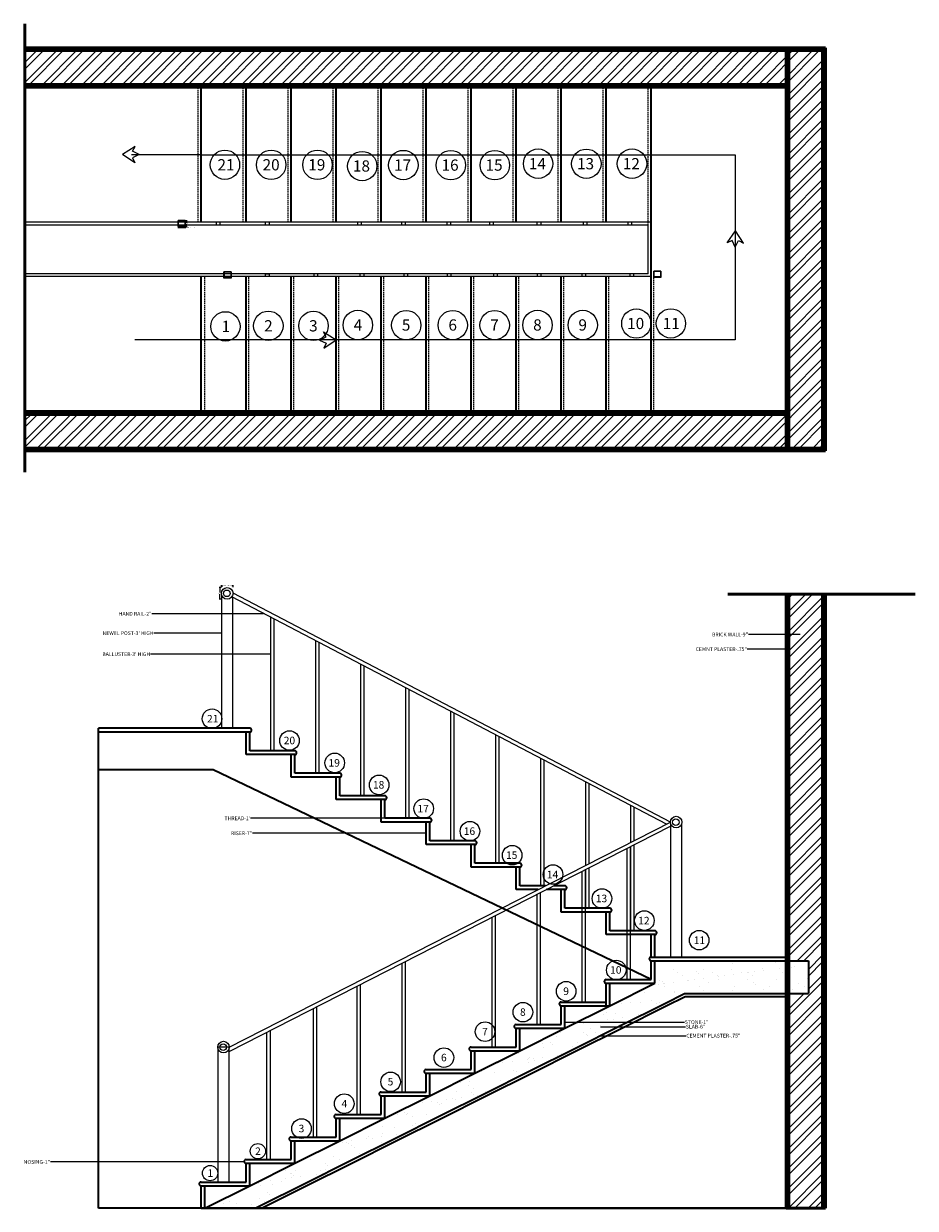
# Model space of a CAD drawing. Units: inches. Extents: x 197 to 435, y -182 to 133.
import ezdxf
from ezdxf import colors
from ezdxf.entities.mleader import LeaderData, LeaderLine
from ezdxf.math import Vec2, Vec3

# ---------------------------------------------------------------- set-up
doc = ezdxf.new("R2010")
doc.units = ezdxf.units.IN
doc.header["$MEASUREMENT"] = 0
doc.linetypes.add('HIDDEN2', pattern=[0.1875, 0.125, -0.0625])
for name, color, linetype, lineweight in [('A-ANNO-DIMS', 2, 'Continuous', 18), ('A-ANNO-NOTE', 7, 'Continuous', 18), ('A-ANNO-SYMB', 2, 'Continuous', 18), ('A-ANNO-TEXT', 7, 'Continuous', 18), ('A-FLOR-HRAL', 4, 'Continuous', 25), ('A-FLOR-STRS', 3, 'Continuous', 35), ('A-FLOR-STRS-OVHD', 3, 'HIDDEN2', 18), ('A-FLOR-STRS-PATT', 252, 'Continuous', 13), ('A-WALL', 7, 'Continuous', 50), ('A-WALL-PATT', 8, 'Continuous', 13)]:
    doc.layers.add(name, color=color, linetype=linetype, lineweight=lineweight)
doc.styles.get("Standard").update_dxf_attribs({"font": 'arial.ttf'})
doc.dimstyles.get("Standard").update_dxf_attribs({"dimtxt": 0.18, "dimasz": 0.18, "dimexe": 0.18, "dimexo": 0.0625, "dimgap": 0.09, "dimtad": 0, "dimtih": 1, "dimtoh": 1, "dimdec": 4, "dimzin": 0, "dimdsep": 46, "dimtxsty": 'Standard', "dimcen": 0.09, "dimadec": 0, "dimazin": 0, "dimtfac": 1, "dimtdec": 4, "dimtofl": 0, "dimtmove": 0, "dimatfit": 3, "dimfxl": 1, "dimtolj": 1, "dimtzin": 0, "dimarcsym": 0})

# ---------------------------------------------------------------- blocks, each defined once
blk = doc.blocks.new('NEWEL-CAP')
for centre, radius in [((250.22, -139.47), 1.54), ((250.22, -139.47), 1.54), ((250.22, -139.47), 1.54), ((250.22, -139.47), 1.54), ((250.33, -139.47), 0.88), ((250.33, -139.47), 0.88)]:
    blk.add_circle(centre, radius)
blk = doc.blocks.new('NEWEL-POST')
for p, q in [((250.41, 65.6), (250.41, 67.25)), ((252.3, 67.25), (250.41, 67.25)), ((252.2, 67.15), (250.51, 67.15)), ((250.51, 65.7), (250.51, 67.15)), ((252.2, 67.15), (252.2, 65.7)), ((252.3, 67.25), (252.3, 65.6)), ((250.74, 65.6), (250.41, 65.6)), ((250.74, 65.7), (250.51, 65.7)), ((252.2, 65.7), (250.74, 65.7)), ((252.3, 65.6), (250.74, 65.6))]:
    blk.add_line(p, q)
blk = doc.blocks.new('ARROW-WALKLINE')
for p, q in [((3.32, 4.4), (0, 2.25)), ((2.65, 3.09), (3.32, 4.4)), ((3.26, 0), (0, 2.25)), ((4.41, 2.19), (2.62, 1.33)), ((2.62, 1.33), (3.26, 0)), ((4.41, 2.19), (2.65, 3.09))]:
    blk.add_line(p, q)
blk = doc.blocks.new('*D4')
at = {"layer": 'A-ANNO-DIMS', "color": 0, "lineweight": -2, "transparency": 16777216}
for p, q in [((238.21, 79.27), (238.21, 78.87)), ((238.39, 79.05), (239.92, 79.05)), ((240.1, 79.27), (240.1, 78.87)), ((240.1, 79.05), (240.28, 79.05))]:
    blk.add_line(p, q, dxfattribs=at)
at = {"layer": 'A-ANNO-DIMS', "color": 0, "transparency": 16777216}
for points in [[(238.39, 79.08), (238.39, 79.02), (238.21, 79.05)], [(239.92, 79.08), (239.92, 79.02), (240.1, 79.05)]]:
    blk.add_solid(points, dxfattribs=at)
at = {"layer": 'Defpoints', "color": 0, "transparency": 16777216}
for p in [(238.21, 79.34), (240.1, 79.34), (240.1, 79.05)]:
    blk.add_point(p, dxfattribs=at)
at = {"layer": 'A-ANNO-DIMS', "color": 0, "transparency": 16777216, "insert": (241.6, 79.05), "char_height": 0.18, "attachment_point": 5}
blk.add_mtext('\\A1;NEWEL POST 2 TYP.', dxfattribs=at)
blk = doc.blocks.new('*D5')
at = {"layer": 'A-ANNO-DIMS', "color": 0, "lineweight": -2, "transparency": 16777216}
for p, q in [((240.17, 80.98), (240.57, 80.98)), ((240.17, 79.34), (240.57, 79.34)), ((240.39, 80.8), (240.39, 80.34)), ((240.39, 79.52), (240.39, 79.98))]:
    blk.add_line(p, q, dxfattribs=at)
at = {"layer": 'A-ANNO-DIMS', "color": 0, "transparency": 16777216}
for points in [[(240.36, 80.8), (240.42, 80.8), (240.39, 80.98)], [(240.36, 79.52), (240.42, 79.52), (240.39, 79.34)]]:
    blk.add_solid(points, dxfattribs=at)
at = {"layer": 'Defpoints', "color": 0, "transparency": 16777216}
for p in [(240.1, 80.98), (240.1, 79.34), (240.39, 80.98)]:
    blk.add_point(p, dxfattribs=at)
at = {"layer": 'A-ANNO-DIMS', "color": 0, "transparency": 16777216, "insert": (240.39, 80.16), "char_height": 0.18, "attachment_point": 5}
blk.add_mtext('\\A1;2 TYP.', dxfattribs=at)
blk = doc.blocks.new('*D6')
at = {"layer": 'A-ANNO-DIMS', "color": 0, "lineweight": -2, "transparency": 16777216}
for p, q in [((249.74, -16.87), (249.74, -16.29)), ((249.92, -16.47), (250.06, -16.47)), ((252.65, -16.47), (252.52, -16.47)), ((252.83, -16.87), (252.83, -16.29))]:
    blk.add_line(p, q, dxfattribs=at)
at = {"layer": 'A-ANNO-DIMS', "color": 0, "transparency": 16777216}
for points in [[(249.92, -16.44), (249.92, -16.5), (249.74, -16.47)], [(252.65, -16.44), (252.65, -16.5), (252.83, -16.47)]]:
    blk.add_solid(points, dxfattribs=at)
at = {"layer": 'Defpoints', "color": 0, "transparency": 16777216}
for p in [(249.74, -16.47), (249.74, -16.93), (252.83, -16.93)]:
    blk.add_point(p, dxfattribs=at)
at = {"layer": 'A-ANNO-DIMS', "color": 0, "transparency": 16777216, "insert": (251.29, -16.47), "char_height": 0.18, "attachment_point": 5}
blk.add_mtext('\\A1;NEWEL CAP 3 TYP.', dxfattribs=at)
blk = doc.blocks.new('*D7')
at = {"layer": 'A-ANNO-DIMS', "color": 0, "lineweight": -2, "transparency": 16777216}
for p, q in [((249.68, -16.93), (249.1, -16.93)), ((249.28, -17.11), (249.28, -18.29)), ((249.28, -19.84), (249.28, -18.66)), ((249.68, -20.02), (249.1, -20.02))]:
    blk.add_line(p, q, dxfattribs=at)
at = {"layer": 'A-ANNO-DIMS', "color": 0, "transparency": 16777216}
for points in [[(249.25, -17.11), (249.31, -17.11), (249.28, -16.93)], [(249.25, -19.84), (249.31, -19.84), (249.28, -20.02)]]:
    blk.add_solid(points, dxfattribs=at)
at = {"layer": 'Defpoints', "color": 0, "transparency": 16777216}
for p in [(249.74, -16.93), (249.28, -20.02), (249.74, -20.02)]:
    blk.add_point(p, dxfattribs=at)
at = {"layer": 'A-ANNO-DIMS', "color": 0, "transparency": 16777216, "insert": (249.28, -18.47), "char_height": 0.18, "attachment_point": 5}
blk.add_mtext('\\A1;3 TYP.', dxfattribs=at)

msp = doc.modelspace()

# ---------------------------------------------------------------- hatches: boundary and pattern name
at = {"layer": 'A-FLOR-STRS-PATT'}
h = msp.add_hatch(dxfattribs=at)
h.set_pattern_fill('AR-SAND', color=256, scale=3)
h.paths.add_polyline_path([(367.97, -127.84), (373.22, -125.22), (400.29, -125.22), (400.29, -116.47), (365.29, -116.47), (365.29, -122.47), (353.29, -128.47), (341.29, -134.47), (329.29, -140.47), (317.29, -146.47), (305.29, -152.47), (293.29, -158.47), (281.29, -164.47), (269.29, -170.47), (257.29, -176.47), (245.29, -182.47), (258.71, -182.47), (259.97, -181.84), (271.97, -175.84), (283.97, -169.84), (295.97, -163.84), (307.97, -157.84), (319.97, -151.84), (331.97, -145.84), (343.97, -139.84), (355.97, -133.84)])
h.paths.add_polyline_path([(406.27, -116.47), (401.04, -116.47), (401.04, -125.22), (406.27, -125.22), (406.27, -125.12)])
at = {"layer": 'A-WALL-PATT'}
h = msp.add_hatch(dxfattribs=at)
h.set_pattern_fill('ANSI32', color=256, scale=10)
h.paths.add_polyline_path([(410.04, 116.5), (410.04, 126.25), (197.3, 126.25), (197.3, 117.25), (401.04, 117.25), (401.04, 29.25), (197.3, 29.25), (197.3, 20.25), (410.04, 20.25)])
h = msp.add_hatch(dxfattribs=at)
h.set_pattern_fill('ANSI32', color=256, scale=10)
h.paths.add_polyline_path([(410.04, -18.72), (401.04, -18.72), (401.04, -116.47), (406.27, -116.47), (406.27, -125.22), (401.04, -125.22), (401.04, -182.47), (410.04, -182.47)])

# ---------------------------------------------------------------- linework, layer by layer
at = {"layer": 'A-ANNO-SYMB'}
for p, q in [((244.29, 98.5), (225.75, 98.5)), ((244.29, 98.5), (386.73, 98.5)), ((386.73, 98.5), (386.73, 49.13)), ((386.73, 49.13), (226.6, 49.13))]:
    msp.add_line(p, q, dxfattribs=at)
for centre, radius in [((250.67, 95.82), 3.92), ((263, 95.79), 3.92), ((275.35, 95.79), 3.92), ((287.27, 95.46), 3.92), ((298.23, 95.74), 3.92), ((310.89, 95.71), 3.92), ((322.64, 95.71), 3.92), ((334.17, 96.1), 3.92), ((347.02, 96.08), 3.92), ((359.21, 96.1), 3.92), ((286.09, 53.08), 3.92), ((299.01, 53.04), 3.92), ((311.41, 53.06), 3.92), ((322.58, 53.06), 3.92), ((334.01, 53.08), 3.92), ((346.08, 53.08), 3.92), ((360.37, 53.47), 3.92), ((369.58, 53.5), 3.92), ((250.79, 52.71), 3.92), ((262.23, 52.88), 3.92), ((274.27, 52.85), 3.92), ((247.23, -51.92), 2.61), ((267.88, -57.73), 2.61), ((279.94, -63.7), 2.61), ((291.78, -69.56), 2.61), ((303.66, -75.88), 2.61), ((316, -81.91), 2.61), ((327.26, -88.31), 2.61), ((338.14, -93.46), 2.61), ((351.2, -99.87), 2.61), ((362.5, -105.74), 2.61), ((377.12, -110.97), 2.61), ((355.01, -118.93), 2.61), ((341.65, -124.59), 2.61), ((330.12, -130.16), 2.61), ((320.02, -135.37), 2.61), ((309.05, -142.29), 2.61), ((294.84, -148.74), 2.61), ((282.48, -154.57), 2.61), ((271.09, -161.21), 2.61), ((259.46, -167.24), 2.04), ((246.7, -173.09), 2.04)]:
    msp.add_circle(centre, radius, dxfattribs=at)
at = {"layer": 'A-FLOR-HRAL'}
for p, q in [((364.29, 80.5), (197.3, 80.5)), ((363.54, 79.75), (197.3, 79.75)), ((248.38, 79.75), (248.38, 80.5)), ((249.29, 80.5), (249.29, 79.75)), ((261.5, 79.75), (261.5, 80.5)), ((262.42, 80.5), (262.42, 79.75)), ((286.06, 79.75), (286.06, 80.5)), ((286.98, 80.5), (286.98, 79.75)), ((297.83, 79.75), (297.83, 80.5)), ((298.74, 80.5), (298.74, 79.75)), ((309.89, 79.75), (309.89, 80.5)), ((310.81, 80.5), (310.81, 79.75)), ((321.27, 79.75), (321.27, 80.5)), ((322.19, 80.5), (322.19, 79.75)), ((333.94, 79.75), (333.94, 80.5)), ((334.86, 80.5), (334.86, 79.75)), ((346.27, 79.75), (346.27, 80.5)), ((347.19, 80.5), (347.19, 79.75)), ((358.15, 79.75), (358.15, 80.5)), ((359.06, 80.5), (359.06, 79.75)), ((363.54, 66.75), (363.54, 79.75)), ((363.54, 66.75), (197.3, 66.75)), ((261.5, 66), (261.5, 66.75)), ((261.5, 66.75), (262.42, 66.75)), ((262.42, 66.75), (262.42, 66)), ((274.43, 66), (274.43, 66.75)), ((275.35, 66.75), (275.35, 66)), ((286.74, 66), (286.74, 66.75)), ((287.66, 66.75), (287.66, 66)), ((298.45, 66), (298.45, 66.75)), ((299.36, 66.75), (299.36, 66)), ((310, 66), (310, 66.75)), ((310.92, 66.75), (310.92, 66)), ((322.35, 66), (322.35, 66.75)), ((323.27, 66.75), (323.27, 66)), ((334.03, 66), (334.03, 66.75)), ((334.94, 66.75), (334.94, 66)), ((345.91, 66), (345.91, 66.75)), ((346.82, 66.75), (346.82, 66)), ((358.7, 66), (358.7, 66.75)), ((359.62, 66.75), (359.62, 66)), ((364.29, 66), (197.3, 66)), ((249.79, -18.84), (249.79, -54.47)), ((369.45, -79.47), (252.83, -18.47)), ((368.36, -80.03), (252.5, -19.43)), ((252.79, -54.47), (252.79, -19.58)), ((262.79, -24.81), (262.79, -60.46)), ((263.79, -60.46), (263.79, -25.33)), ((274.79, -31.09), (274.79, -66.46)), ((275.79, -66.46), (275.79, -31.61)), ((286.79, -37.36), (286.79, -72.46)), ((287.79, -72.46), (287.79, -37.89)), ((298.79, -43.64), (298.79, -78.46)), ((299.79, -78.46), (299.79, -44.16)), ((310.79, -49.92), (310.79, -84.46)), ((311.79, -84.46), (311.79, -50.44)), ((322.79, -56.19), (322.79, -90.46)), ((323.79, -90.46), (323.79, -56.72)), ((334.79, -62.47), (334.79, -96.46)), ((335.79, -96.46), (335.79, -62.99)), ((346.79, -68.75), (346.79, -91.04)), ((347.79, -90.53), (347.79, -69.27)), ((358.79, -75.02), (358.79, -84.91)), ((359.79, -84.4), (359.79, -75.55)), ((251.79, -140.62), (369.5, -80.57)), ((251.83, -139.47), (369.45, -79.47)), ((369.5, -79.84), (369.5, -115.47)), ((372.5, -115.47), (372.5, -79.84)), ((357.79, -86.55), (357.79, -121.46)), ((358.79, -121.46), (358.79, -86.04)), ((358.79, -86.04), (358.79, -108.46)), ((359.79, -108.46), (359.79, -85.53)), ((345.79, -92.67), (345.79, -127.46)), ((346.79, -127.46), (346.79, -92.16)), ((346.79, -92.16), (346.79, -102.46)), ((347.79, -102.46), (347.79, -91.65)), ((333.79, -98.79), (333.79, -133.46)), ((334.79, -133.46), (334.79, -98.28)), ((321.79, -104.91), (321.79, -139.46)), ((322.79, -139.46), (322.79, -104.4)), ((298.79, -151.46), (298.79, -116.64)), ((297.79, -117.15), (297.79, -151.46)), ((286.79, -157.46), (286.79, -122.76)), ((285.79, -123.27), (285.79, -157.46)), ((274.17, -129.2), (274.17, -163.46)), ((275.17, -163.46), (275.17, -128.69)), ((261.79, -135.52), (261.79, -169.46)), ((262.79, -169.46), (262.79, -135.01)), ((251.79, -139.47), (248.79, -139.47)), ((248.79, -139.47), (248.79, -175.47)), ((251.79, -175.47), (251.79, -139.47)), ((262.29, -169.47), (262.79, -169.46)), ((250.29, -175.47), (251.79, -175.47))]:
    msp.add_line(p, q, dxfattribs=at)
at = {"layer": 'A-FLOR-STRS'}
for p, q in [((244.29, 80.5), (244.29, 116.5)), ((256.29, 80.5), (256.29, 116.5)), ((268.29, 80.5), (268.29, 116.5)), ((280.29, 80.5), (280.29, 116.5)), ((292.29, 80.5), (292.29, 116.5)), ((304.29, 80.5), (304.29, 116.5)), ((316.29, 80.5), (316.29, 116.5)), ((328.29, 80.5), (328.29, 116.5)), ((340.29, 80.5), (340.29, 116.5)), ((352.29, 80.5), (352.29, 116.5)), ((364.29, 66.75), (364.29, 116.5)), ((364.29, 30), (364.29, 66.75)), ((244.29, 30), (244.29, 66)), ((256.29, 30), (256.29, 66)), ((268.29, 30), (268.29, 66)), ((280.29, 30), (280.29, 66)), ((292.29, 30), (292.29, 66)), ((304.29, 30), (304.29, 66)), ((316.29, 30), (316.29, 66)), ((328.29, 30), (328.29, 66)), ((340.29, 30), (340.29, 66)), ((352.29, 30), (352.29, 66)), ((257.29, -54.47), (216.98, -54.47)), ((216.98, -182.47), (216.98, -54.47)), ((257.29, -55.47), (216.98, -55.47)), ((256.29, -61.47), (256.29, -55.47)), ((257.29, -60.47), (257.29, -55.47)), ((269.29, -61.47), (256.29, -61.47)), ((269.29, -60.47), (257.29, -60.47)), ((268.29, -67.47), (268.29, -61.47)), ((269.29, -66.47), (269.29, -61.47)), ((247.49, -65.55), (216.98, -65.55)), ((364.29, -121.47), (247.49, -65.55)), ((281.29, -67.47), (268.29, -67.47)), ((281.29, -66.47), (269.29, -66.47)), ((280.29, -73.47), (280.29, -67.47)), ((281.29, -72.47), (281.29, -67.47)), ((293.29, -72.47), (281.29, -72.47)), ((293.29, -73.47), (280.29, -73.47)), ((292.29, -79.47), (292.29, -73.47)), ((293.29, -78.47), (293.29, -73.47)), ((305.29, -78.47), (293.29, -78.47)), ((305.29, -79.47), (292.29, -79.47)), ((304.29, -85.47), (304.29, -79.47)), ((305.29, -84.47), (305.29, -79.47)), ((317.29, -84.47), (305.29, -84.47)), ((317.29, -85.47), (304.29, -85.47)), ((316.29, -91.47), (316.29, -85.47)), ((317.29, -90.47), (317.29, -85.47)), ((329.29, -91.47), (316.29, -91.47)), ((329.29, -90.47), (317.29, -90.47)), ((328.29, -97.47), (328.29, -91.47)), ((329.29, -96.47), (329.29, -91.47)), ((334.17, -97.47), (328.29, -97.47)), ((336.13, -96.47), (329.29, -96.47)), ((341.29, -97.47), (336.37, -97.47)), ((341.29, -96.47), (338.33, -96.47)), ((340.29, -103.47), (340.29, -97.47)), ((341.29, -102.47), (341.29, -97.47)), ((353.29, -103.47), (340.29, -103.47)), ((353.29, -102.47), (341.29, -102.47)), ((352.29, -109.47), (352.29, -103.47)), ((353.29, -108.47), (353.29, -103.47)), ((365.29, -109.47), (352.29, -109.47)), ((365.29, -108.47), (353.29, -108.47)), ((364.29, -115.47), (364.29, -109.47)), ((365.29, -115.47), (365.29, -109.47)), ((364.29, -115.47), (400.29, -115.47)), ((364.29, -121.47), (364.29, -116.47)), ((364.29, -116.47), (400.29, -116.47)), ((365.29, -122.47), (365.29, -116.47)), ((400.29, -116.47), (406.27, -116.47)), ((406.27, -116.47), (406.27, -125.12)), ((352.29, -121.47), (364.29, -121.47)), ((352.29, -128.47), (352.29, -122.47)), ((352.29, -122.47), (365.29, -122.47)), ((353.29, -128.47), (353.29, -122.47)), ((353.29, -128.47), (365.29, -122.47)), ((367.97, -127.84), (373.22, -125.22)), ((368.31, -128.51), (373.4, -125.97)), ((373.22, -125.22), (400.29, -125.22)), ((373.4, -125.97), (400.29, -125.97)), ((400.29, -125.22), (406.27, -125.22)), ((406.27, -125.22), (406.27, -125.12)), ((340.29, -127.47), (352.29, -127.47)), ((340.29, -133.47), (340.29, -128.47)), ((340.29, -128.47), (353.29, -128.47)), ((341.29, -134.47), (341.29, -128.47)), ((341.29, -134.47), (353.29, -128.47)), ((355.97, -133.84), (367.97, -127.84)), ((356.31, -134.51), (368.31, -128.51)), ((328.29, -133.47), (340.29, -133.47)), ((328.29, -139.47), (328.29, -134.47)), ((328.29, -134.47), (341.29, -134.47)), ((329.29, -140.47), (329.29, -134.47)), ((329.29, -140.47), (341.29, -134.47)), ((343.97, -139.84), (355.97, -133.84)), ((344.31, -140.51), (356.31, -134.51)), ((316.29, -139.47), (328.29, -139.47)), ((316.29, -145.47), (316.29, -140.47)), ((316.29, -140.47), (329.29, -140.47)), ((317.29, -146.47), (317.29, -140.47)), ((317.29, -146.47), (329.29, -140.47)), ((331.97, -145.84), (343.97, -139.84)), ((332.31, -146.51), (344.31, -140.51)), ((304.29, -145.47), (316.29, -145.47)), ((304.29, -151.47), (304.29, -146.47)), ((304.29, -146.47), (317.29, -146.47)), ((305.29, -152.47), (305.29, -146.47)), ((305.29, -152.47), (317.29, -146.47)), ((319.97, -151.84), (331.97, -145.84)), ((320.31, -152.51), (332.31, -146.51)), ((292.29, -151.47), (304.29, -151.47)), ((292.29, -157.47), (292.29, -152.47)), ((292.29, -152.47), (305.29, -152.47)), ((293.29, -158.47), (293.29, -152.47)), ((293.29, -158.47), (305.29, -152.47)), ((307.97, -157.84), (319.97, -151.84)), ((308.31, -158.51), (320.31, -152.51)), ((280.29, -157.47), (292.29, -157.47)), ((295.97, -163.84), (307.97, -157.84)), ((280.29, -163.47), (280.29, -158.47)), ((280.29, -158.47), (293.29, -158.47)), ((281.29, -164.47), (281.29, -158.47)), ((281.29, -164.47), (293.29, -158.47)), ((296.31, -164.51), (308.31, -158.51)), ((268.29, -163.47), (280.29, -163.47)), ((283.97, -169.84), (295.97, -163.84)), ((268.29, -169.47), (268.29, -164.47)), ((268.29, -164.47), (281.29, -164.47)), ((269.29, -170.47), (269.29, -164.47)), ((269.29, -170.47), (281.29, -164.47)), ((284.31, -170.51), (296.31, -164.51)), ((256.29, -169.47), (268.29, -169.47)), ((256.29, -175.47), (256.29, -170.47)), ((256.29, -170.47), (269.29, -170.47)), ((257.29, -176.47), (257.29, -170.47)), ((257.29, -176.47), (269.29, -170.47)), ((271.97, -175.84), (283.97, -169.84)), ((272.31, -176.51), (284.31, -170.51)), ((244.29, -175.47), (256.29, -175.47)), ((244.29, -182.47), (244.29, -176.47)), ((244.29, -176.47), (257.29, -176.47)), ((245.29, -182.47), (245.29, -176.47)), ((245.29, -182.47), (257.29, -176.47)), ((259.97, -181.84), (271.97, -175.84)), ((260.38, -182.47), (272.31, -176.51)), ((400.29, -182.47), (216.98, -182.47)), ((244.29, -182.47), (400.29, -182.47)), ((258.71, -182.47), (259.97, -181.84))]:
    msp.add_line(p, q, dxfattribs=at)
for centre, start, end in [((257.29, -54.97), 270, 90), ((269.29, -60.97), 270, 90), ((281.29, -66.97), 270, 90), ((293.29, -72.97), 270, 90), ((305.29, -78.97), 270, 90), ((317.29, -84.97), 270, 90), ((329.29, -90.97), 270, 90), ((341.29, -96.97), 270, 90), ((353.29, -102.97), 270, 90), ((365.29, -108.97), 270, 90), ((364.29, -115.97), 90, 270), ((352.29, -121.97), 90, 270), ((340.29, -127.97), 90, 270), ((328.29, -133.97), 90, 270), ((316.29, -139.97), 90, 270), ((304.29, -145.97), 90, 270), ((292.29, -151.97), 90, 270), ((280.29, -157.97), 90, 270), ((268.29, -163.97), 90, 270), ((256.29, -169.97), 90, 270), ((244.29, -175.97), 90, 270)]:
    msp.add_arc(centre, 0.5, start, end, dxfattribs=at)
at = {"layer": 'A-FLOR-STRS-OVHD', "ltscale": 3}
for p, q in [((243.54, 80.5), (243.54, 116.5)), ((255.54, 80.5), (255.54, 116.5)), ((267.54, 80.5), (267.54, 116.5)), ((279.54, 80.5), (279.54, 116.5)), ((291.54, 80.5), (291.54, 116.5)), ((303.54, 80.5), (303.54, 116.5)), ((315.54, 80.5), (315.54, 116.5)), ((327.54, 80.5), (327.54, 116.5)), ((339.54, 80.5), (339.54, 116.5)), ((351.54, 80.5), (351.54, 116.5)), ((363.54, 66.75), (363.54, 116.5)), ((365.04, 30), (365.04, 66.75)), ((245.29, 30), (245.29, 66)), ((257.04, 30), (257.04, 66)), ((269.04, 30), (269.04, 66)), ((281.04, 30), (281.04, 66)), ((293.04, 30), (293.04, 66)), ((305.04, 30), (305.04, 66)), ((317.04, 30), (317.04, 66)), ((329.04, 30), (329.04, 66)), ((341.04, 30), (341.04, 66)), ((353.04, 30), (353.04, 66))]:
    msp.add_line(p, q, dxfattribs=at)
at = {"layer": 'A-WALL'}
for p, q in [((197.3, 133.43), (197.3, 13.82)), ((410.79, 127), (197.3, 127)), ((400.29, 19.5), (400.29, 127)), ((401.04, 19.5), (401.04, 127)), ((410.04, 19.5), (410.04, 127)), ((410.79, 117.25), (410.79, 127)), ((410.79, 19.5), (410.79, 127)), ((410.04, 126.25), (197.3, 126.25)), ((410.04, 116.5), (410.04, 126.25)), ((401.04, 117.25), (197.3, 117.25)), ((401.04, 29.25), (401.04, 117.25)), ((410.79, 19.5), (410.79, 117.25)), ((400.29, 116.5), (197.3, 116.5)), ((400.29, 30), (400.29, 116.5)), ((410.04, 20.25), (410.04, 116.5)), ((400.29, 30), (197.3, 30)), ((401.04, 29.25), (197.3, 29.25)), ((410.04, 20.25), (197.3, 20.25)), ((410.79, 19.5), (197.3, 19.5)), ((384.75, -18.72), (434.75, -18.72)), ((400.29, -182.47), (400.29, -18.72)), ((401.04, -182.47), (401.04, -18.72)), ((410.04, -182.47), (410.04, -18.72)), ((410.79, -182.47), (410.79, -18.72)), ((400.29, -182.47), (410.79, -182.47))]:
    msp.add_line(p, q, dxfattribs=at)

# ---------------------------------------------------------------- block references
at = {"layer": 'A-ANNO-SYMB'}
msp.add_blockref('ARROW-WALKLINE', (223.38, 96.32), dxfattribs=at)
for p, rotation in [((384.55, 78.23), 269.9999999999994), ((280.22, 51.37), 181.813157911352)]:
    msp.add_blockref('ARROW-WALKLINE', p, dxfattribs=dict(at, rotation=rotation))
at = {"layer": 'A-FLOR-HRAL'}
for p in [(-12.2, 13.73), (0, 0), (114.63, 0.19)]:
    msp.add_blockref('NEWEL-POST', p, dxfattribs=at)
at = {"layer": 'A-FLOR-HRAL', "rotation": 180}
for p in [(501.5, -157.95), (621.21, -218.95), (500.5, -278.95)]:
    msp.add_blockref('NEWEL-CAP', p, dxfattribs=at)

# ---------------------------------------------------------------- texts
at = {"layer": 'A-ANNO-TEXT'}
for s, height, p in [('21', 3, (248.67, 94.31)), ('20', 3, (260.71, 94.31)), ('19', 3, (272.89, 94.31)), ('18', 3, (284.8, 93.98)), ('17', 3, (295.77, 94.23)), ('16', 3, (308.43, 94.23)), ('15', 3, (320.16, 94.23)), ('14', 3, (331.71, 94.6)), ('13', 3, (344.55, 94.6)), ('12', 3, (356.76, 94.6)), ('1', 3, (249.78, 51.2)), ('2', 3, (261.12, 51.37)), ('3', 3, (273.11, 51.37)), ('4', 3, (285, 51.58)), ('5', 3, (297.84, 51.58)), ('6', 3, (310.26, 51.58)), ('7', 3, (321.41, 51.58)), ('8', 3, (332.85, 51.6)), ('9', 3, (344.92, 51.6)), ('10', 3, (357.91, 51.99)), ('11', 3, (367.4, 51.99)), ('21', 2, (245.89, -52.92)), ('20', 2, (266.35, -58.72)), ('19', 2, (278.29, -64.68)), ('18', 2, (290.13, -70.55)), ('17', 2, (302.02, -76.88)), ('16', 2, (314.35, -82.9)), ('15 ', 2, (325.61, -89.29)), ('14', 2, (336.5, -94.47)), ('13', 2, (349.56, -100.85)), ('12', 2, (360.87, -106.74)), ('11', 2, (375.67, -111.98)), ('10', 2, (353.37, -119.91)), ('9', 2, (340.88, -125.58)), ('8', 2, (329.34, -131.15)), ('7', 2, (319.24, -136.36)), ('6', 2, (308.28, -143.27)), ('5', 2, (294.06, -149.71)), ('4', 2, (281.76, -155.57)), ('3', 2, (270.32, -162.2)), ('2', 2, (258.71, -168.24)), ('1', 2, (246.02, -174.09))]:
    msp.add_text(s, height=height, dxfattribs=at).set_placement(p)

# ---------------------------------------------------------------- dimensions: what is measured, and where the dimension line sits
at = {"layer": 'A-ANNO-DIMS'}
dim = msp.add_linear_dim(base=(240.1, 79.05), p1=(238.21, 79.34), p2=(240.1, 79.34), text='NEWEL POST <> TYP.', dimstyle='Standard', override={"dimdec": 0, "dimlfac": 1, "dimrnd": 0, "dimzin": 0, "dimdsep": 46, "dimlunit": 2}, dxfattribs=at)
dim.commit()
dim.dimension.update_dxf_attribs({"geometry": '*D4', "text_midpoint": (241.6, 79.05)})
for base, p1, p2, angle, text, picture, middle in [((240.39, 80.98), (240.1, 79.34), (240.1, 80.98), 90, '<> TYP.', '*D5', (240.39, 80.16)), ((249.28, -20.02), (249.74, -16.93), (249.74, -20.02), 270, '<> TYP.', '*D7', (249.28, -18.47)), ((249.74, -16.47), (252.83, -16.93), (249.74, -16.93), 180, 'NEWEL CAP <> TYP.', '*D6', (251.29, -16.47))]:
    dim = msp.add_linear_dim(base=base, p1=p1, p2=p2, angle=angle, text=text, dimstyle='Standard', override={"dimdec": 0, "dimlfac": 1, "dimrnd": 0, "dimzin": 0, "dimdsep": 46, "dimlunit": 2}, dxfattribs=at)
    dim.commit()
    dim.dimension.update_dxf_attribs({"geometry": picture, "text_midpoint": middle})

# ---------------------------------------------------------------- leaders
at = {"layer": 'A-ANNO-NOTE'}
ml = msp.add_multileader_mtext('Standard', dxfattribs=at)
ml.set_content('HAND RAIL-2"', color=256)
ml.set_leader_properties()
ml.build(insert=Vec2(0, 0))
ml.multileader.update_dxf_attribs({"dogleg_length": 0.36, "arrow_head_size": 0.18})
ctx = ml.context
ctx.base_point, ctx.char_height, ctx.arrow_head_size, ctx.landing_gap_size, ctx.plane_origin = Vec3(222.01, -23.92), 1, 0.18, 0.09, Vec3(261.09, -23.92)
ctx.text_align_type = 2
notes = []
notes.append((ctx, [(0, (1, 1, 0), (231.57, -23.92), (-1, 0), 0.36, [(0, [(261.09, -23.92)], 0, [])])]))
ctx.mtext.insert, ctx.mtext.alignment, ctx.mtext.flow_direction = Vec3(231.12, -23.42), 3, 5
ml = msp.add_multileader_mtext('Standard', dxfattribs=at)
ml.set_content("NEWEL POST-3' HIGH", color=256)
ml.set_leader_properties()
ml.build(insert=Vec2(0, 0))
ml.multileader.update_dxf_attribs({"dogleg_length": 0.36, "arrow_head_size": 0.18})
ctx = ml.context
ctx.base_point, ctx.char_height, ctx.arrow_head_size, ctx.landing_gap_size, ctx.plane_origin = Vec3(217.2, -29.09), 1, 0.18, 0.09, Vec3(249.79, -29.09)
ctx.text_align_type = 2
notes.append((ctx, [(0, (1, 1, 0), (232.07, -29.09), (-1, 0), 0.36, [(0, [(249.79, -29.09)], 0, [])])]))
ctx.mtext.insert, ctx.mtext.alignment, ctx.mtext.flow_direction = Vec3(231.62, -28.58), 3, 5
ml = msp.add_multileader_mtext('Standard', dxfattribs=at)
ml.set_content('BRICK WALL-9"', color=256)
ml.set_leader_properties()
ml.build(insert=Vec2(0, 0))
ml.multileader.update_dxf_attribs({"dogleg_length": 0.36, "arrow_head_size": 0.18})
ctx = ml.context
ctx.base_point, ctx.char_height, ctx.arrow_head_size, ctx.landing_gap_size, ctx.plane_origin = Vec3(380.02, -29.47), 1, 0.18, 0.09, Vec3(404.21, -29.47)
ctx.text_align_type = 2
notes.append((ctx, [(0, (1, 1, 0), (390.59, -29.47), (-1, 0), 0.36, [(0, [(404.21, -29.47)], 0, [])])]))
ctx.mtext.insert, ctx.mtext.alignment, ctx.mtext.flow_direction = Vec3(390.14, -28.96), 3, 5
ml = msp.add_multileader_mtext('Standard', dxfattribs=at)
ml.set_content("BALLUSTER-3' HIGH ", color=256)
ml.set_leader_properties()
ml.build(insert=Vec2(0, 0))
ml.multileader.update_dxf_attribs({"dogleg_length": 0.36, "arrow_head_size": 0.18})
ctx = ml.context
ctx.base_point, ctx.char_height, ctx.arrow_head_size, ctx.landing_gap_size, ctx.plane_origin = Vec3(217.3, -34.7), 1, 0.18, 0.09, Vec3(262.79, -34.7)
ctx.text_align_type = 2
notes.append((ctx, [(0, (1, 1, 0), (231.16, -34.7), (-1, 0), 0.36, [(0, [(262.79, -34.7)], 0, [])])]))
ctx.mtext.insert, ctx.mtext.alignment, ctx.mtext.flow_direction = Vec3(230.71, -34.19), 3, 5
ml = msp.add_multileader_mtext('Standard', dxfattribs=at)
ml.set_content('CEMNT PLASTER-.75"', color=256)
ml.set_leader_properties()
ml.build(insert=Vec2(0, 0))
ml.multileader.update_dxf_attribs({"dogleg_length": 0.36, "arrow_head_size": 0.18})
ctx = ml.context
ctx.base_point, ctx.char_height, ctx.arrow_head_size, ctx.landing_gap_size, ctx.plane_origin = Vec3(375.25, -33.37), 1, 0.18, 0.09, Vec3(400.29, -33.37)
ctx.text_align_type = 2
notes.append((ctx, [(0, (1, 1, 0), (390.28, -33.37), (-1, 0), 0.36, [(0, [(400.29, -33.37)], 0, [])])]))
ctx.mtext.insert, ctx.mtext.alignment, ctx.mtext.flow_direction = Vec3(389.83, -32.86), 3, 5
ml = msp.add_multileader_mtext('Standard', dxfattribs=at)
ml.set_content("THREAD-1'", color=256)
ml.set_leader_properties()
ml.build(insert=Vec2(0, 0))
ml.multileader.update_dxf_attribs({"dogleg_length": 0.36, "arrow_head_size": 0.18})
ctx = ml.context
ctx.base_point, ctx.char_height, ctx.arrow_head_size, ctx.landing_gap_size, ctx.plane_origin = Vec3(250.16, -78.47), 1, 0.18, 0.09, Vec3(296.72, -78.47)
ctx.text_align_type = 2
notes.append((ctx, [(0, (1, 1, 0), (257.86, -78.47), (-1, 0), 0.36, [(0, [(296.72, -78.47)], 0, [])])]))
ctx.mtext.insert, ctx.mtext.alignment, ctx.mtext.flow_direction = Vec3(257.41, -77.97), 3, 5
ml = msp.add_multileader_mtext('Standard', dxfattribs=at)
ml.set_content('RISER-7"', color=256)
ml.set_leader_properties()
ml.build(insert=Vec2(0, 0))
ml.multileader.update_dxf_attribs({"dogleg_length": 0.36, "arrow_head_size": 0.18})
ctx = ml.context
ctx.base_point, ctx.char_height, ctx.arrow_head_size, ctx.landing_gap_size, ctx.plane_origin = Vec3(251.99, -82.47), 1, 0.18, 0.09, Vec3(304.29, -82.47)
ctx.text_align_type = 2
notes.append((ctx, [(0, (1, 1, 0), (258.36, -82.47), (-1, 0), 0.36, [(0, [(304.29, -82.47)], 0, [])])]))
ctx.mtext.insert, ctx.mtext.alignment, ctx.mtext.flow_direction = Vec3(257.91, -81.96), 3, 5
ml = msp.add_multileader_mtext('Standard', dxfattribs=at)
ml.set_content('STONE-1"', color=256)
ml.set_leader_properties()
ml.build(insert=Vec2(0, 0))
ml.multileader.update_dxf_attribs({"dogleg_length": 0.36, "arrow_head_size": 0.18})
ctx = ml.context
ctx.base_point, ctx.char_height, ctx.arrow_head_size, ctx.landing_gap_size, ctx.plane_origin = Vec3(373.22, -132.82), 1, 0.18, 0.09, Vec3(340.86, -132.82)
notes.append((ctx, [(0, (1, 1, 0), (372.86, -132.82), (1, 0), 0.36, [(0, [(340.86, -132.82)], 0, [])])]))
ctx.mtext.insert, ctx.mtext.flow_direction = Vec3(373.31, -132.31), 5
ml = msp.add_multileader_mtext('Standard', dxfattribs=at)
ml.set_content('SLAB-6"', color=256)
ml.set_leader_properties()
ml.build(insert=Vec2(0, 0))
ml.multileader.update_dxf_attribs({"dogleg_length": 3, "arrow_head_size": 0.18})
ctx = ml.context
ctx.base_point, ctx.char_height, ctx.arrow_head_size, ctx.landing_gap_size, ctx.plane_origin = Vec3(373.49, -134.05), 1, 0.18, 0.09, Vec3(350.61, -134.05)
notes.append((ctx, [(0, (1, 1, 0), (370.49, -134.05), (1, 0), 3, [(0, [(350.61, -134.05)], 0, [])])]))
ctx.mtext.insert, ctx.mtext.flow_direction = Vec3(373.58, -133.54), 5
ml = msp.add_multileader_mtext('Standard', dxfattribs=at)
ml.set_content('CEMENT PLASTER-.75"', color=256)
ml.set_leader_properties()
ml.build(insert=Vec2(0, 0))
ml.multileader.update_dxf_attribs({"dogleg_length": 0.36, "arrow_head_size": 0.18})
ctx = ml.context
ctx.base_point, ctx.char_height, ctx.arrow_head_size, ctx.landing_gap_size, ctx.plane_origin = Vec3(373.58, -136.44), 1, 0.18, 0.09, Vec3(350.77, -136.44)
notes.append((ctx, [(0, (1, 1, 0), (373.22, -136.44), (1, 0), 0.36, [(0, [(350.77, -136.44)], 0, [])])]))
ctx.mtext.insert, ctx.mtext.flow_direction = Vec3(373.67, -135.93), 5
ml = msp.add_multileader_mtext('Standard', dxfattribs=at)
ml.set_content('NOSING-1"', color=256)
ml.set_leader_properties()
ml.build(insert=Vec2(0, 0))
ml.multileader.update_dxf_attribs({"dogleg_length": 0.36, "arrow_head_size": 0.18})
ctx = ml.context
ctx.base_point, ctx.char_height, ctx.arrow_head_size, ctx.landing_gap_size, ctx.plane_origin = Vec3(196.85, -170.12), 1, 0.18, 0.09, Vec3(255.81, -170.12)
ctx.text_align_type = 2
notes.append((ctx, [(0, (1, 1, 0), (204.47, -170.12), (-1, 0), 0.36, [(0, [(255.81, -170.12)], 0, [])])]))
ctx.mtext.insert, ctx.mtext.alignment, ctx.mtext.flow_direction = Vec3(204.02, -169.61), 3, 5
for ctx, leaders in notes:
    for number, flags, end, landing, length, lines in leaders:
        leader = LeaderData()
        leader.index, (leader.has_last_leader_line, leader.has_dogleg_vector, leader.attachment_direction) = number, flags
        leader.last_leader_point, leader.dogleg_vector, leader.dogleg_length = Vec3(end), Vec3(landing), length
        for number, points, colour, breaks in lines:
            line = LeaderLine()
            line.index, line.vertices, line.color, line.breaks = number, Vec3.list(points), colors.encode_raw_color(colour), breaks
            leader.lines.append(line)
        ctx.leaders.append(leader)

doc.saveas('drawing.dxf')
